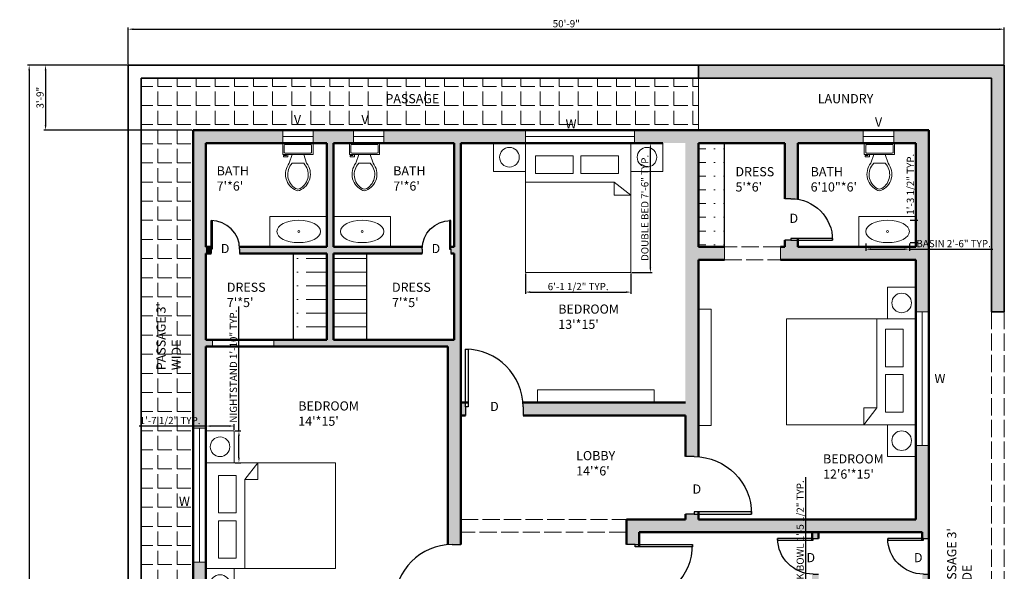
# Model space of a CAD drawing. Units: inches. Extents: x 554 to 1300, y 1707 to 2873.
# Tile 3 of 3: x 554 to 1238, y 2490 to 2873. Entities that reach past the tile are written whole.
import ezdxf

# ---------------------------------------------------------------- set-up
doc = ezdxf.new("R2010")
doc.units = ezdxf.units.IN
doc.linetypes.add('ACAD_ISO02W100', pattern=[15, 12, -3])
for name, color, linetype, lineweight in [('A-ANNO-DIMS', 145, 'Continuous', 18), ('A-AREA-IDEN', 145, 'Continuous', 25), ('A-CASE', 8, 'Continuous', 25), ('A-CASE-PATT', 245, 'Continuous', 13), ('A-FLOR-FIXT', 9, 'Continuous', 18), ('A-WALL-OVHD', 30, 'ACAD_ISO02W100', 18), ('A-WALL-PATT', 30, 'Continuous', 13), ('C-PROP', 30, 'Continuous', 35), ('C-PROP-OVHD', 30, 'ACAD_ISO02W100', 18), ('C-PVMT', 8, 'Continuous', 18), ('C-PVMT-PATT', 116, 'Continuous', 13), ('DOOR', 52, 'Continuous', 25), ('FUR', 210, 'Continuous', 18), ('TEXT', 145, 'Continuous', 18), ('WALL', 30, 'Continuous', 50), ('WIND', 70, 'Continuous', 18)]:
    doc.layers.add(name, color=color, linetype=linetype, lineweight=lineweight)
doc.styles.get("Standard").update_dxf_attribs({"font": 'arial.ttf'})
doc.dimstyles.new('ISO-25', dxfattribs={"dimtxt": 5, "dimasz": 3.5, "dimexe": 1.25, "dimexo": 0.625, "dimtad": 1, "dimdec": 0, "dimlunit": 4, "dimtxsty": 'Standard', "dimcen": 2.5, "dimadec": 0, "dimazin": 0, "dimtfac": 1, "dimtdec": 0, "dimtmove": 0, "dimatfit": 3, "dimfxl": 1, "dimarcsym": 0})

# ---------------------------------------------------------------- blocks, each defined once
blk = doc.blocks.new('*U2')
for p, q in [((0, 0), (0, -6)), ((40, 0), (40, -6))]:
    blk.add_line(p, q)
blk.add_lwpolyline([(0, 0), (0, 40), (1.75, 40), (1.75, 0)], close=True)
blk.add_arc((0, 0), 40, 0, 90)
blk = doc.blocks.new('*U4')
for p, q in [((9.5, -6), (9.5, -2)), ((-10, -8.5), (-8, -8.5)), ((-10, -9.5), (-10, -8.5)), ((-7, -9.5), (-10, -9.5)), ((-8, -8.5), (-8, -8)), ((-7, -8), (-7, -9.5)), ((-4, -8), (-6, -14)), ((4, -8), (6, -14)), ((4, -14), (-4, -14))]:
    blk.add_line(p, q)
blk.add_lwpolyline([(10.5, -8), (10.5, 0), (-10.5, 0), (-10.5, -8)], close=True)
for points in [[(-9.5, -2), (-9.5, -6)], [(8.5, -1), (-8.5, -1)], [(-8.5, -7), (8.5, -7)]]:
    blk.add_lwpolyline(points)
for centre, radius, start, end in [((-8.62, -1.88), 0.884, 81.8699, 188.1301), ((-8.62, -6.12), 0.884, 171.8699, 278.1301), ((8.62, -1.88), 0.884, 351.8699, 98.1301), ((8.62, -6.12), 0.884, 261.8699, 8.1301), ((3.52, -21.58), 12.17, 141.46911, 247.97143), ((4.2, -21.82), 11.33, 136.36773, 238.94682), ((-3.52, -21.58), 12.17, 292.02843, 38.53071), ((-4.2, -21.82), 11.33, 301.05301, 43.63209), ((0, -27.88), 4, 245.73182, 294.26817), ((0, -29), 4, 254.86053, 285.13947)]:
    blk.add_arc(centre, radius, start, end)
blk = doc.blocks.new('*D7')
at = {"layer": 'A-ANNO-DIMS', "color": 0, "lineweight": -2, "transparency": 16777216}
for p, q in [((629.68, 2842.1), (629.68, 2867.75)), ((633.18, 2866.5), (1234.68, 2866.5)), ((1238.18, 2842.1), (1238.18, 2867.75))]:
    blk.add_line(p, q, dxfattribs=at)
at = {"layer": 'A-ANNO-DIMS', "color": 0, "lineweight": 100, "transparency": 16777216}
for points in [[(633.18, 2867.08), (633.18, 2865.92), (629.68, 2866.5)], [(1234.68, 2867.08), (1234.68, 2865.92), (1238.18, 2866.5)]]:
    blk.add_solid(points, dxfattribs=at)
at = {"layer": 'Defpoints', "color": 0, "lineweight": 100, "transparency": 16777216}
for p in [(1238.18, 2866.5), (629.68, 2841.48), (1238.18, 2841.48)]:
    blk.add_point(p, dxfattribs=at)
at = {"layer": 'A-ANNO-DIMS', "color": 0, "transparency": 16777216, "insert": (933.93, 2869.68), "char_height": 5, "attachment_point": 5}
blk.add_mtext('50\'-9"', dxfattribs=at)
blk = doc.blocks.new('*D8')
at = {"layer": 'A-ANNO-DIMS', "color": 0, "lineweight": -2, "transparency": 16777216}
for p, q in [((629.06, 2841.48), (559.64, 2841.48)), ((560.89, 2837.98), (560.89, 1770.98)), ((629.06, 1767.48), (559.64, 1767.48))]:
    blk.add_line(p, q, dxfattribs=at)
at = {"layer": 'A-ANNO-DIMS', "color": 0, "lineweight": 100, "transparency": 16777216}
for points in [[(560.3, 2837.98), (561.47, 2837.98), (560.89, 2841.48)], [(560.3, 1770.98), (561.47, 1770.98), (560.89, 1767.48)]]:
    blk.add_solid(points, dxfattribs=at)
at = {"layer": 'Defpoints', "color": 0, "lineweight": 100, "transparency": 16777216}
for p in [(629.68, 2841.48), (560.89, 1767.48), (629.68, 1767.48)]:
    blk.add_point(p, dxfattribs=at)
at = {"layer": 'A-ANNO-DIMS', "color": 0, "transparency": 16777216, "insert": (557.71, 2304.48), "char_height": 5, "attachment_point": 5, "rotation": 90}
blk.add_mtext('89\'-6"', dxfattribs=at)
blk = doc.blocks.new('BED-DOUBLE')
for p, q in [((0, 62.82), (61.67, 62.82)), ((61.67, 62.82), (61.67, 53.82)), ((73.37, 53.82), (61.67, 62.82)), ((61.67, 53.82), (73.37, 53.82))]:
    blk.add_line(p, q)
blk.add_lwpolyline([(73.37, 89.87), (73.37, 0), (0, 0), (0, 89.87)])
for points in [[(7.06, 81.16), (33.12, 81.16), (33.12, 68.85), (7.06, 68.85)], [(38.57, 81.16), (64.63, 81.16), (64.63, 68.85), (38.57, 68.85)]]:
    blk.add_lwpolyline(points, close=True)
blk = doc.blocks.new('NIGHTSTAND')
blk.add_lwpolyline([(22.14, 19.58), (0, 19.58), (0, 0), (22.14, 0)], close=True)
blk.add_circle((11.07, 9.79), 6.79)
blk = doc.blocks.new('BASIN-OVAL')
blk.add_circle((15.12, 7.78), 0.687)
blk.add_ellipse((15.12, 7.78), major_axis=(15.12, 0), ratio=0.514491)
blk = doc.blocks.new('*D18')
at = {"layer": 'A-ANNO-DIMS', "color": 0, "lineweight": -2, "transparency": 16777216}
for p, q in [((706.58, 2587.89), (706.58, 2674.1)), ((703.88, 2587.89), (707.83, 2587.89)), ((706.58, 2569.25), (706.58, 2584.39)), ((703.88, 2565.75), (707.83, 2565.75))]:
    blk.add_line(p, q, dxfattribs=at)
at = {"layer": 'A-ANNO-DIMS', "color": 0, "lineweight": 100, "transparency": 16777216}
for points in [[(706, 2584.39), (707.16, 2584.39), (706.58, 2587.89)], [(706, 2569.25), (707.16, 2569.25), (706.58, 2565.75)]]:
    blk.add_solid(points, dxfattribs=at)
at = {"layer": 'Defpoints', "color": 0, "lineweight": 100, "transparency": 16777216}
for p in [(703.26, 2587.89), (706.58, 2587.89), (703.26, 2565.75)]:
    blk.add_point(p, dxfattribs=at)
at = {"layer": 'A-ANNO-DIMS', "color": 0, "transparency": 16777216, "insert": (703.37, 2632.74), "char_height": 5, "attachment_point": 5, "rotation": 90}
blk.add_mtext('NIGHTSTAND 1\'-10" TYP.', dxfattribs=at)
blk = doc.blocks.new('*D19')
at = {"layer": 'A-ANNO-DIMS', "color": 0, "lineweight": -2, "transparency": 16777216}
for p, q in [((683.68, 2588.51), (683.68, 2592.46)), ((703.26, 2588.51), (703.26, 2592.46)), ((683.68, 2591.21), (637.27, 2591.21)), ((699.76, 2591.21), (687.18, 2591.21))]:
    blk.add_line(p, q, dxfattribs=at)
at = {"layer": 'A-ANNO-DIMS', "color": 0, "lineweight": 100, "transparency": 16777216}
for points in [[(687.18, 2591.79), (687.18, 2590.62), (683.68, 2591.21)], [(699.76, 2591.79), (699.76, 2590.62), (703.26, 2591.21)]]:
    blk.add_solid(points, dxfattribs=at)
at = {"layer": 'Defpoints', "color": 0, "lineweight": 100, "transparency": 16777216}
for p in [(683.68, 2591.21), (683.68, 2587.89), (703.26, 2587.89)]:
    blk.add_point(p, dxfattribs=at)
at = {"layer": 'A-ANNO-DIMS', "color": 0, "transparency": 16777216, "insert": (658.73, 2594.42), "char_height": 5, "attachment_point": 5}
blk.add_mtext('1\'-7 1/2" TYP.', dxfattribs=at)
blk = doc.blocks.new('*D22')
at = {"layer": 'A-ANNO-DIMS', "color": 0, "lineweight": -2, "transparency": 16777216}
for p, q in [((1142.01, 2717.81), (1142.01, 2712.65)), ((1172.26, 2717.81), (1172.26, 2712.65)), ((1145.51, 2713.9), (1168.76, 2713.9)), ((1172.26, 2713.9), (1230.16, 2713.9))]:
    blk.add_line(p, q, dxfattribs=at)
at = {"layer": 'A-ANNO-DIMS', "color": 0, "lineweight": 100, "transparency": 16777216}
for points in [[(1145.51, 2714.48), (1145.51, 2713.32), (1142.01, 2713.9)], [(1168.76, 2714.48), (1168.76, 2713.32), (1172.26, 2713.9)]]:
    blk.add_solid(points, dxfattribs=at)
at = {"layer": 'Defpoints', "color": 0, "lineweight": 100, "transparency": 16777216}
for p in [(1142.01, 2718.44), (1172.26, 2718.44), (1172.26, 2713.9)]:
    blk.add_point(p, dxfattribs=at)
at = {"layer": 'A-ANNO-DIMS', "color": 0, "transparency": 16777216, "insert": (1202.96, 2717.11), "char_height": 5, "attachment_point": 5}
blk.add_mtext('BASIN 2\'-6" TYP.', dxfattribs=at)
blk = doc.blocks.new('*D23')
at = {"layer": 'A-ANNO-DIMS', "color": 0, "lineweight": -2, "transparency": 16777216}
for p, q in [((1176.79, 2734), (1176.79, 2780.41)), ((1172.88, 2734), (1178.04, 2734)), ((1176.79, 2721.94), (1176.79, 2730.5)), ((1172.88, 2718.44), (1178.04, 2718.44))]:
    blk.add_line(p, q, dxfattribs=at)
at = {"layer": 'A-ANNO-DIMS', "color": 0, "lineweight": 100, "transparency": 16777216}
for points in [[(1176.21, 2730.5), (1177.38, 2730.5), (1176.79, 2734)], [(1176.21, 2721.94), (1177.38, 2721.94), (1176.79, 2718.44)]]:
    blk.add_solid(points, dxfattribs=at)
at = {"layer": 'Defpoints', "color": 0, "lineweight": 100, "transparency": 16777216}
for p in [(1172.26, 2734), (1176.79, 2734), (1172.26, 2718.44)]:
    blk.add_point(p, dxfattribs=at)
at = {"layer": 'A-ANNO-DIMS', "color": 0, "transparency": 16777216, "insert": (1173.58, 2758.95), "char_height": 5, "attachment_point": 5, "rotation": 90}
blk.add_mtext('1\'-3 1/2" TYP.', dxfattribs=at)
blk = doc.blocks.new('*D24')
at = {"layer": 'A-ANNO-DIMS', "color": 0, "lineweight": -2, "transparency": 16777216}
for p, q in [((979.52, 2787.48), (993.62, 2787.48)), ((992.37, 2701.11), (992.37, 2783.98)), ((979.52, 2697.61), (993.62, 2697.61))]:
    blk.add_line(p, q, dxfattribs=at)
at = {"layer": 'A-ANNO-DIMS', "color": 0, "lineweight": 100, "transparency": 16777216}
for points in [[(991.79, 2783.98), (992.96, 2783.98), (992.37, 2787.48)], [(991.79, 2701.11), (992.96, 2701.11), (992.37, 2697.61)]]:
    blk.add_solid(points, dxfattribs=at)
at = {"layer": 'Defpoints', "color": 0, "lineweight": 100, "transparency": 16777216}
for p in [(978.89, 2787.48), (992.37, 2787.48), (978.89, 2697.61)]:
    blk.add_point(p, dxfattribs=at)
at = {"layer": 'A-ANNO-DIMS', "color": 0, "transparency": 16777216, "insert": (989.16, 2742.54), "char_height": 5, "attachment_point": 5, "rotation": 90}
blk.add_mtext('DOUBLE BED 7\'-6" TYP.', dxfattribs=at)
blk = doc.blocks.new('*D25')
at = {"layer": 'A-ANNO-DIMS', "color": 0, "lineweight": -2, "transparency": 16777216}
for p, q in [((905.53, 2696.98), (905.53, 2682.87)), ((978.89, 2696.98), (978.89, 2682.87)), ((909.03, 2684.12), (975.39, 2684.12))]:
    blk.add_line(p, q, dxfattribs=at)
at = {"layer": 'A-ANNO-DIMS', "color": 0, "lineweight": 100, "transparency": 16777216}
for points in [[(909.03, 2684.71), (909.03, 2683.54), (905.53, 2684.12)], [(975.39, 2684.71), (975.39, 2683.54), (978.89, 2684.12)]]:
    blk.add_solid(points, dxfattribs=at)
at = {"layer": 'Defpoints', "color": 0, "lineweight": 100, "transparency": 16777216}
for p in [(905.53, 2697.61), (978.89, 2697.61), (978.89, 2684.12)]:
    blk.add_point(p, dxfattribs=at)
at = {"layer": 'A-ANNO-DIMS', "color": 0, "transparency": 16777216, "insert": (942.21, 2687.33), "char_height": 5, "attachment_point": 5}
blk.add_mtext('6\'-1 1/2" TYP.', dxfattribs=at)
blk = doc.blocks.new('*D28')
at = {"layer": 'A-ANNO-DIMS', "color": 0, "lineweight": -2, "transparency": 16777216}
for p, q in [((1100.29, 2468.04), (1100.29, 2555.65)), ((1098.27, 2468.04), (1101.54, 2468.04)), ((1100.29, 2453.96), (1100.29, 2464.54)), ((1098.27, 2450.46), (1101.54, 2450.46))]:
    blk.add_line(p, q, dxfattribs=at)
at = {"layer": 'A-ANNO-DIMS', "color": 0, "lineweight": 100, "transparency": 16777216}
for points in [[(1099.7, 2464.54), (1100.87, 2464.54), (1100.29, 2468.04)], [(1099.7, 2453.96), (1100.87, 2453.96), (1100.29, 2450.46)]]:
    blk.add_solid(points, dxfattribs=at)
at = {"layer": 'Defpoints', "color": 0, "lineweight": 100, "transparency": 16777216}
for p in [(1097.65, 2468.04), (1100.29, 2468.04), (1097.65, 2450.46)]:
    blk.add_point(p, dxfattribs=at)
at = {"layer": 'A-ANNO-DIMS', "color": 0, "transparency": 16777216, "insert": (1097.07, 2513.59), "char_height": 5, "attachment_point": 5, "rotation": 90}
blk.add_mtext('SINK BOWL 1\'-5 1/2" TYP.', dxfattribs=at)
blk = doc.blocks.new('*D35')
at = {"layer": 'A-ANNO-DIMS', "color": 0, "lineweight": -2, "transparency": 16777216}
for p, q in [((629.06, 2841.48), (571.03, 2841.48)), ((572.28, 2837.98), (572.28, 2799.98)), ((674.06, 2796.48), (571.03, 2796.48))]:
    blk.add_line(p, q, dxfattribs=at)
at = {"layer": 'A-ANNO-DIMS', "color": 0, "lineweight": 100, "transparency": 16777216}
for points in [[(571.7, 2837.98), (572.86, 2837.98), (572.28, 2841.48)], [(571.7, 2799.98), (572.86, 2799.98), (572.28, 2796.48)]]:
    blk.add_solid(points, dxfattribs=at)
at = {"layer": 'Defpoints', "color": 0, "lineweight": 100, "transparency": 16777216}
for p in [(629.68, 2841.48), (572.28, 2796.48), (674.68, 2796.48)]:
    blk.add_point(p, dxfattribs=at)
at = {"layer": 'A-ANNO-DIMS', "color": 0, "transparency": 16777216, "insert": (569.1, 2818.98), "char_height": 5, "attachment_point": 5, "rotation": 90}
blk.add_mtext('3\'-9"', dxfattribs=at)

msp = doc.modelspace()

# ---------------------------------------------------------------- hatches: boundary and pattern name
at = {"layer": 'A-CASE-PATT'}
h = msp.add_hatch(dxfattribs=at)
h.set_pattern_fill('ACAD_ISO04W100', color=256, scale=1.9)
h.paths.add_polyline_path([(767.68, 2710.98), (744.53, 2710.98), (744.53, 2650.98), (767.68, 2650.98)])
h.paths.add_polyline_path([(795.22, 2710.98), (772.18, 2710.98), (772.18, 2650.98), (795.22, 2650.98)])
h.paths.add_polyline_path([(1043.78, 2787.48), (1025.68, 2787.48), (1025.68, 2715.48), (1043.78, 2715.48)])
at = {"layer": 'A-WALL-PATT'}
h = msp.add_hatch(color=256, dxfattribs=at)
h.dxf.hatch_style = 1
h.paths.add_polyline_path([(1238.18, 2841.48), (1025.68, 2841.48), (1025.68, 2832.48), (1229.18, 2832.48), (1229.18, 2670.52), (1238.18, 2670.52)])
h = msp.add_hatch(color=256, dxfattribs=at)
h.dxf.hatch_style = 1
h.paths.add_polyline_path([(1136.18, 2067.48), (1026.18, 2067.48), (1026.18, 2065.48), (1134.18, 2065.48), (1134.18, 2039.48), (1026.18, 2039.48), (1026.18, 2037.48), (1136.18, 2037.48)])
h.paths.add_polyline_path([(1193.18, 2103.48), (1184.18, 2103.48), (1184.18, 2077.52), (1193.18, 2077.52)])
h.paths.add_polyline_path([(1193.18, 2032.94), (1184.18, 2032.94), (1184.18, 2001.48), (1148.18, 2001.48), (1136.18, 2001.48), (1128.74, 2001.48), (1128.74, 1992.48), (1193.18, 1992.48), (1193.18, 2001.48)])
h.paths.add_polyline_path([(1076.18, 2001.48), (1045.59, 2001.48), (1045.59, 1992.48), (1076.18, 1992.48)])
h.paths.add_polyline_path([(993.02, 2001.48), (923.53, 2001.48), (923.53, 1996.9), (923.53, 1992.48), (993.02, 1992.48)])
h.paths.add_polyline_path([(1184.18, 2112.48), (962.18, 2112.48), (962.18, 2151.15), (953.18, 2151.15), (953.18, 2103.48), (1184.18, 2103.48)])
h.paths.add_polyline_path([(1193.18, 2144.33), (1184.18, 2144.33), (1184.18, 2112.48), (1184.18, 2103.48), (1193.18, 2103.48)])
h.paths.add_polyline_path([(772.18, 2796.48), (758.22, 2796.48), (758.22, 2787.48), (767.68, 2787.48), (772.18, 2787.48)])
h.paths.add_polyline_path([(737.06, 2796.48), (674.68, 2796.48), (674.68, 2710.98), (683.68, 2710.98), (683.68, 2715.48), (683.68, 2787.48), (737.06, 2787.48)])
h.paths.add_polyline_path([(786.15, 2796.48), (772.18, 2796.48), (772.18, 2787.48), (786.15, 2787.48)])
h.paths.add_polyline_path([(860.68, 2796.48), (807.31, 2796.48), (807.31, 2787.48), (856.18, 2787.48), (860.68, 2787.48)])
h.paths.add_polyline_path([(905.53, 2796.48), (860.68, 2796.48), (860.68, 2787.48), (905.53, 2787.48)])
h.paths.add_polyline_path([(860.68, 2787.48), (856.18, 2787.48), (856.18, 2715.48), (853.67, 2715.48), (853.67, 2713.96), (853.67, 2710.98), (856.18, 2710.98), (860.68, 2710.98)])
h.paths.add_polyline_path([(772.18, 2787.48), (767.68, 2787.48), (767.68, 2715.48), (728.12, 2715.48), (706.98, 2715.48, -0.019152), (707.04, 2713.96), (707.04, 2710.98), (772.18, 2710.98)])
h.paths.add_polyline_path([(833.86, 2715.48), (772.18, 2715.48), (772.18, 2710.98), (833.8, 2710.98), (833.8, 2713.96, -0.019152)])
h.paths.add_polyline_path([(1025.68, 2796.48), (981.39, 2796.48), (981.39, 2787.48), (1001.03, 2787.48), (1016.68, 2787.48), (1025.68, 2787.48)])
h.paths.add_polyline_path([(1094.68, 2796.48), (1025.68, 2796.48), (1025.68, 2787.48), (1085.68, 2787.48), (1094.68, 2787.48)])
h.paths.add_polyline_path([(1140.18, 2796.48), (1094.68, 2796.48), (1094.68, 2787.48), (1140.18, 2787.48)], flags=17)
h.paths.add_polyline_path([(1185.68, 2796.48), (1161.35, 2796.48), (1161.35, 2787.48), (1176.68, 2787.48), (1176.68, 2736.68), (1176.72, 2736.68), (1176.72, 2715.48), (1137.16, 2715.48), (1094.68, 2715.48), (1094.68, 2706.48), (1185.68, 2706.48)])
h.paths.add_polyline_path([(1094.68, 2787.48), (1085.68, 2787.48), (1085.68, 2748.92), (1090.01, 2748.92, -0.040642), (1094.68, 2748.54)])
h.paths.add_polyline_path([(1025.68, 2787.48), (1016.68, 2787.48), (1016.68, 2607.48), (1016.68, 2598.48), (1025.68, 2598.48), (1025.68, 2672.36), (1025.68, 2706.48)])
h.paths.add_polyline_path([(1094.68, 2715.48), (1094.68, 2720.05), (1090.01, 2720.05), (1085.68, 2720.05), (1085.68, 2715.48), (1082.66, 2715.48), (1082.66, 2706.48), (1094.68, 2706.48)])
h.paths.add_polyline_path([(1043.78, 2715.48), (1025.68, 2715.48), (1025.68, 2706.48), (1043.78, 2706.48)])
h.paths.add_polyline_path([(1185.68, 2577.7), (1176.68, 2577.7), (1176.68, 2570), (1176.68, 2526.48), (1176.68, 2517.48), (1185.68, 2517.48)])
h.paths.add_polyline_path([(1185.68, 2706.48), (1176.68, 2706.48), (1176.68, 2670.52), (1185.68, 2670.52)])
h.paths.add_polyline_path([(1025.68, 2598.48), (1016.68, 2598.48), (1016.68, 2569.99), (1022.68, 2569.99, -0.01877), (1025.68, 2569.88)])
h.paths.add_polyline_path([(1016.68, 2607.48), (903.83, 2607.48, -0.01877), (903.94, 2604.48), (903.94, 2598.48), (1016.68, 2598.48)])
h.paths.add_polyline_path([(860.68, 2646.48), (851.68, 2646.48), (851.68, 2508.85, -0.01877), (854.68, 2508.96), (860.68, 2508.96)])
h.paths.add_polyline_path([(863.94, 2604.48), (863.94, 2607.48), (860.68, 2607.48), (860.68, 2598.48), (863.94, 2598.48)])
h.paths.add_polyline_path([(1101.44, 2750.41), (1134.65, 2750.41), (1134.65, 2774.1), (1101.44, 2774.1)], flags=25)
h.paths.add_polyline_path([(1049.21, 2750.31), (1082.94, 2750.31), (1082.94, 2773.99), (1049.21, 2773.99)], flags=9)
h = msp.add_hatch(color=256, dxfattribs=at)
h.dxf.hatch_style = 1
h.paths.add_polyline_path([(687.18, 2713.96), (687.18, 2715.48), (683.68, 2715.48), (683.68, 2710.98), (687.18, 2710.98)])
h = msp.add_hatch(color=256, dxfattribs=at)
h.dxf.hatch_style = 1
h.paths.add_polyline_path([(683.68, 2710.98), (674.68, 2710.98), (674.68, 2646.48), (674.68, 2589.67), (683.68, 2589.67), (683.68, 2646.48), (683.68, 2650.98)])
h.paths.add_polyline_path([(688.17, 2650.98), (683.68, 2650.98), (683.68, 2646.48), (688.17, 2646.48)])
h.paths.add_polyline_path([(772.18, 2710.98), (767.68, 2710.98), (767.68, 2650.98), (730.85, 2650.98), (730.85, 2646.48), (772.18, 2646.48)])
h.paths.add_polyline_path([(860.68, 2710.98), (856.18, 2710.98), (856.18, 2650.98), (772.18, 2650.98), (772.18, 2646.48), (860.68, 2646.48)])
h.paths.add_polyline_path([(683.68, 2496.84), (674.68, 2496.84), (674.68, 2445.48), (683.68, 2445.48), (683.68, 2454.48)])
h.paths.add_polyline_path([(851.68, 2454.48), (683.68, 2454.48), (683.68, 2445.48), (851.68, 2445.48)])
h.paths.add_polyline_path([(707.68, 2445.48), (698.68, 2445.48), (698.68, 2419.1), (707.68, 2419.1)])
h.paths.add_polyline_path([(698.68, 2289.48), (687.57, 2289.48), (687.57, 2280.48), (696.57, 2280.48), (698.68, 2280.48)])
h.paths.add_polyline_path([(687.57, 2217.48), (671.17, 2217.48), (671.17, 2208.48), (687.57, 2208.48)])
h.paths.add_polyline_path([(650.01, 2217.48), (638.68, 2217.48), (638.68, 2208.48), (650.01, 2208.48)])
h.paths.add_polyline_path([(860.68, 2235.34), (854.68, 2235.34, -0.01877), (851.68, 2235.45), (851.68, 2112.48), (696.57, 2112.48), (696.57, 2103.48), (860.68, 2103.48)])
h.paths.add_polyline_path([(666.88, 1959.48), (647.68, 1959.48), (638.68, 1959.48), (638.68, 1950.48), (647.68, 1950.48), (666.88, 1950.48)])
h.paths.add_polyline_path([(756.66, 1959.48), (719.44, 1959.48), (719.44, 1950.48), (756.66, 1950.48)])
h.paths.add_polyline_path([(860.68, 1992.48), (864.62, 1992.48), (864.62, 1996.9), (864.62, 2001.48), (860.68, 2001.48), (860.68, 2058.13), (854.68, 2058.13, -0.01877), (851.68, 2058.24), (851.68, 1992.48), (851.68, 1959.48), (809.22, 1959.48), (809.22, 1950.48), (860.68, 1950.48)])
h.paths.add_polyline_path([(860.68, 2103.48), (851.68, 2103.48), (851.68, 2098.13), (854.68, 2098.13), (860.68, 2098.13)])
h.paths.add_polyline_path([(984.68, 2397.2), (984.68, 2469.19, -0.01877), (981.68, 2469.08), (975.68, 2469.08), (975.68, 2361.48), (975.68, 2355.65), (984.68, 2355.65), (984.68, 2361.48), (984.68, 2370.48)])
h.paths.add_polyline_path([(1109.18, 2409.48), (1104.68, 2409.48), (1104.68, 2370.48), (984.68, 2370.48), (984.68, 2361.48), (1109.18, 2361.48)])
h.paths.add_polyline_path([(1125.26, 2418.48), (1109.18, 2418.48), (1109.18, 2488.51), (1105.47, 2488.51, -0.008003), (1104.68, 2488.52), (1104.68, 2409.48), (1109.18, 2409.48), (1125.26, 2409.48)])
h.paths.add_polyline_path([(1185.68, 2418.48), (1167, 2418.48), (1167, 2409.48), (1185.68, 2409.48)])
h.paths.add_polyline_path([(1185.68, 2488.51), (1181.97, 2488.51, -0.008003), (1181.18, 2488.52), (1181.18, 2418.48), (1185.68, 2418.48)])
h.paths.add_polyline_path([(1025.68, 2529.99), (1022.68, 2529.99), (1016.68, 2529.99), (1016.68, 2526.48), (975.68, 2526.48), (975.68, 2517.48), (1025.68, 2517.48)])
h.paths.add_polyline_path([(984.68, 2517.48), (975.68, 2517.48), (975.68, 2509.08), (981.68, 2509.08), (984.68, 2509.08)])
h.paths.add_polyline_path([(1176.68, 2526.48), (1025.68, 2526.48), (1025.68, 2517.48), (1104.68, 2517.48), (1176.68, 2517.48)])
h.paths.add_polyline_path([(745.17, 1864.25), (773.96, 1864.25), (773.96, 1877.33), (745.17, 1877.33)], flags=9)
h = msp.add_hatch(color=256, dxfattribs=at)
h.dxf.hatch_style = 1
h.paths.add_polyline_path([(638.68, 2072.33), (638.68, 2103.48), (638.68, 2217.48), (629.68, 2217.48), (629.68, 2097.48), (629.68, 1992.48), (629.68, 1950.48), (638.68, 1950.48), (638.68, 1992.48)])
h.paths.add_polyline_path([(696.57, 2217.48), (687.57, 2217.48), (687.57, 2142.07, -0.048021), (692.61, 2142.55), (696.57, 2142.55)])
h.paths.add_polyline_path([(696.57, 2116.14), (692.61, 2116.14), (687.57, 2116.14), (687.57, 2112.48), (638.68, 2112.48), (638.68, 2103.48), (687.57, 2103.48), (696.57, 2103.48), (696.57, 2112.48)])
h.paths.add_polyline_path([(1010.14, 2078.06), (1025.63, 2078.06), (1025.63, 2091.14), (1010.14, 2091.14)], flags=9)
h.paths.add_polyline_path([(1129.91, 2440.07), (1172.04, 2440.07), (1172.04, 2474.45), (1129.91, 2474.45)], flags=9)
h.paths.add_polyline_path([(1022.04, 2432.2), (1064.45, 2432.2), (1064.45, 2455.89), (1022.04, 2455.89)], flags=9)
h.paths.add_polyline_path([(891.25, 2147.87), (936.31, 2147.87), (936.31, 2182.23), (891.25, 2182.23)], flags=9)
h.paths.add_polyline_path([(951.1, 2040.21), (1005.03, 2040.21), (1005.03, 2063.9), (951.1, 2063.9)], flags=9)
h.paths.add_polyline_path([(988, 1912.76), (1023.48, 1912.76), (1023.48, 1936.45), (988, 1936.45)], flags=9)
h.paths.add_polyline_path([(735.06, 2044.01), (781.37, 2044.01), (781.37, 2078.39), (735.06, 2078.39)], flags=9)
h.paths.add_polyline_path([(651.07, 2140.85), (677.89, 2140.85), (677.89, 2164.54), (651.07, 2164.54)], flags=9)
h.paths.add_polyline_path([(769.16, 2219.79), (818.47, 2219.79), (818.47, 2243.48), (769.16, 2243.48)], flags=9)
h.paths.add_polyline_path([(745.28, 2587.79), (794.59, 2587.79), (794.59, 2611.48), (745.28, 2611.48)], flags=9)
h = msp.add_hatch(color=256, dxfattribs=at)
h.dxf.hatch_style = 1
h.paths.add_polyline_path([(1109.18, 2517.48), (1104.68, 2517.48), (1104.68, 2513.23), (1105.47, 2513.23), (1109.18, 2513.23)])
h.paths.add_polyline_path([(1185.68, 2517.48), (1181.18, 2517.48), (1181.18, 2513.23), (1181.97, 2513.23), (1185.68, 2513.23)])
at = {"layer": 'C-PVMT-PATT'}
h = msp.add_hatch(dxfattribs=at)
h.set_pattern_fill('ANGLE', color=256, scale=1.9)
h.set_pattern_definition([(0, (0, 0), (0, 13.2715), [9.652, -3.6195]), (90, (0, 0), (-13.2715, 8e-16), [9.652, -3.6195])])
h.paths.add_polyline_path([(674.68, 2646.48), (674.68, 2710.98), (674.68, 2796.48), (772.18, 2796.48), (860.68, 2796.48), (1025.68, 2796.48), (1025.68, 2832.48), (638.68, 2832.48), (638.68, 2217.48), (674.68, 2217.48), (674.68, 2445.48)])

# ---------------------------------------------------------------- linework, layer by layer
at = {"layer": 'A-CASE'}
for p, q in [((1043.78, 2715.48), (1043.78, 2787.48)), ((744.53, 2650.98), (744.53, 2710.98)), ((795.22, 2710.98), (795.22, 2650.98))]:
    msp.add_line(p, q, dxfattribs=at)
at = {"layer": 'A-FLOR-FIXT'}
for points in [[(767.68, 2715.48), (728.12, 2715.48), (728.12, 2736.68), (767.68, 2736.68)], [(811.74, 2715.48), (772.18, 2715.48), (772.18, 2736.68), (811.74, 2736.68)], [(1176.72, 2715.48), (1137.16, 2715.48), (1137.16, 2736.68), (1176.72, 2736.68)]]:
    msp.add_lwpolyline(points, close=True, dxfattribs=at)
at = {"layer": 'A-WALL-OVHD'}
for points in [[(1043.78, 2706.48), (1043.78, 2715.48)], [(1082.66, 2715.48), (1082.66, 2706.48)]]:
    msp.add_lwpolyline(points, dxfattribs=at)
for points in [[(1043.78, 2706.48), (1082.66, 2706.48), (1082.66, 2715.48), (1043.78, 2715.48)], [(688.17, 2650.98), (730.85, 2650.98), (730.85, 2646.48), (688.17, 2646.48)], [(975.68, 2517.48), (860.68, 2517.48), (860.68, 2526.48), (975.68, 2526.48)]]:
    msp.add_lwpolyline(points, close=True, dxfattribs=at)
at = {"layer": 'C-PROP'}
for p, q in [((629.68, 2841.48), (629.68, 2097.48)), ((629.68, 2841.48), (1238.18, 2841.48)), ((1025.68, 2832.48), (1025.68, 2841.48)), ((1238.18, 2670.52), (1238.18, 2841.48)), ((638.68, 2832.48), (1229.18, 2832.48)), ((638.68, 2832.48), (638.68, 2097.48)), ((1229.18, 2670.52), (1229.18, 2832.48)), ((1229.18, 2670.52), (1238.18, 2670.52))]:
    msp.add_line(p, q, dxfattribs=at)
at = {"layer": 'C-PROP-OVHD'}
msp.add_lwpolyline([(1229.18, 2418.48), (1238.18, 2418.48), (1238.18, 2670.52), (1229.18, 2670.52)], close=True, dxfattribs=at)
at = {"layer": 'C-PVMT'}
msp.add_line((1025.68, 2796.48), (1025.68, 2832.48), dxfattribs=at)
at = {"layer": 'FUR'}
for p, q in [((719.73, 2565.75), (710.74, 2554.05)), ((719.73, 2554.05), (719.73, 2565.75)), ((710.74, 2492.38), (710.74, 2554.05)), ((710.74, 2554.05), (719.73, 2554.05))]:
    msp.add_line(p, q, dxfattribs=at)
for points in [[(1001.03, 2787.48), (978.89, 2787.48), (978.89, 2767.9), (1001.03, 2767.9)], [(1025.68, 2672.36), (1025.68, 2591.51), (1034.61, 2591.51), (1034.61, 2672.36)], [(914.03, 2607.48), (994.88, 2607.48), (994.88, 2616.41), (914.03, 2616.41)], [(1176.68, 2570), (1176.68, 2592.14), (1157.1, 2592.14), (1157.1, 2570)], [(692.39, 2530.95), (692.39, 2557.01), (704.7, 2557.01), (704.7, 2530.95)], [(692.39, 2499.44), (692.39, 2525.5), (704.7, 2525.5), (704.7, 2499.44)]]:
    msp.add_lwpolyline(points, close=True, dxfattribs=at)
msp.add_lwpolyline([(683.68, 2565.75), (773.56, 2565.75), (773.56, 2492.38), (683.68, 2492.38), (683.68, 2496.84)], dxfattribs=at)
for centre in [(989.96, 2777.69), (1166.89, 2581.07)]:
    msp.add_circle(centre, 6.79, dxfattribs=at)
at = {"layer": 'WALL'}
for p, q in [((674.68, 2796.48), (772.18, 2796.48)), ((674.68, 2710.98), (674.68, 2796.48)), ((772.18, 2796.48), (860.68, 2796.48)), ((860.68, 2796.48), (1025.68, 2796.48)), ((1025.68, 2796.48), (1094.68, 2796.48)), ((1094.68, 2796.48), (1185.68, 2796.48)), ((1185.68, 2796.48), (1185.68, 2706.48)), ((683.68, 2787.48), (767.68, 2787.48)), ((683.68, 2715.48), (683.68, 2787.48)), ((767.68, 2787.48), (767.68, 2715.48)), ((772.18, 2787.48), (772.18, 2715.48)), ((772.18, 2787.48), (856.18, 2787.48)), ((856.18, 2787.48), (856.18, 2715.48)), ((860.68, 2787.48), (860.68, 2710.98)), ((860.68, 2787.48), (1001.03, 2787.48)), ((1025.68, 2787.48), (1025.68, 2715.48)), ((1025.68, 2787.48), (1085.68, 2787.48)), ((1085.68, 2787.48), (1085.68, 2748.92)), ((1094.68, 2787.48), (1094.68, 2748.54)), ((1094.68, 2787.48), (1176.68, 2787.48)), ((1176.68, 2787.48), (1176.68, 2715.48)), ((688.05, 2715.48), (683.68, 2715.48)), ((767.68, 2715.48), (706.98, 2715.48)), ((833.86, 2715.48), (772.18, 2715.48)), ((856.18, 2715.48), (852.8, 2715.48)), ((1043.78, 2715.48), (1025.68, 2715.48)), ((1085.68, 2715.48), (1082.66, 2715.48)), ((1085.68, 2720.05), (1085.68, 2715.48)), ((1094.68, 2721.31), (1094.68, 2715.48)), ((1176.68, 2715.48), (1094.68, 2715.48)), ((674.68, 2710.98), (674.68, 2646.48)), ((683.68, 2710.98), (683.68, 2650.98)), ((687.18, 2710.98), (683.68, 2710.98)), ((767.68, 2710.98), (707.04, 2710.98)), ((767.68, 2650.98), (767.68, 2710.98)), ((772.18, 2650.98), (772.18, 2710.98)), ((772.18, 2710.98), (833.8, 2710.98)), ((833.8, 2710.98), (772.18, 2710.98)), ((856.18, 2710.98), (853.67, 2710.98)), ((853.67, 2710.98), (856.18, 2710.98)), ((856.18, 2710.98), (856.18, 2650.98)), ((860.68, 2710.98), (860.68, 2646.48)), ((1025.68, 2706.48), (1025.68, 2569.88)), ((1043.78, 2706.48), (1025.68, 2706.48)), ((1025.68, 2706.48), (1025.68, 2598.48)), ((1094.68, 2706.48), (1082.66, 2706.48)), ((1176.68, 2706.48), (1094.68, 2706.48)), ((1176.68, 2526.48), (1176.68, 2706.48)), ((1185.68, 2517.48), (1185.68, 2706.48)), ((683.68, 2650.98), (767.68, 2650.98)), ((856.18, 2650.98), (772.18, 2650.98)), ((674.68, 2646.48), (674.68, 2445.48)), ((683.68, 2646.48), (772.18, 2646.48)), ((683.68, 2646.48), (683.68, 2454.48)), ((851.68, 2646.48), (772.18, 2646.48)), ((851.68, 2508.85), (851.68, 2646.48)), ((860.68, 2508.96), (860.68, 2646.48)), ((865.69, 2607.48), (860.68, 2607.48)), ((1016.68, 2607.48), (903.83, 2607.48)), ((860.68, 2598.48), (860.68, 2526.48)), ((863.94, 2598.48), (860.68, 2598.48)), ((1016.68, 2598.48), (903.94, 2598.48)), ((1016.68, 2598.48), (1016.68, 2569.99)), ((1025.68, 2598.48), (1025.68, 2569.88)), ((1025.68, 2531.74), (1025.68, 2526.48)), ((1025.68, 2531.74), (1025.68, 2526.48)), ((1016.68, 2526.48), (975.68, 2526.48)), ((975.68, 2517.48), (975.68, 2526.48)), ((1016.68, 2529.99), (1016.68, 2526.48)), ((1025.68, 2526.48), (1176.68, 2526.48)), ((975.68, 2517.48), (975.68, 2509.08)), ((1025.68, 2517.48), (984.68, 2517.48)), ((1104.68, 2517.48), (984.68, 2517.48)), ((984.68, 2517.48), (984.68, 2507.33)), ((1025.68, 2517.48), (1181.18, 2517.48)), ((1104.68, 2512.15), (1104.68, 2517.48)), ((1109.18, 2513.23), (1109.18, 2517.48)), ((1181.18, 2517.48), (1181.18, 2512.15)), ((1185.68, 2517.48), (1185.68, 2418.48))]:
    msp.add_line(p, q, dxfattribs=at)
at = {"layer": 'WIND'}
for p, q in [((737.06, 2791.98), (758.22, 2791.98)), ((786.15, 2791.98), (807.31, 2791.98)), ((905.53, 2791.98), (981.39, 2791.98)), ((1140.18, 2791.98), (1161.35, 2791.98)), ((1181.18, 2577.7), (1181.18, 2670.52)), ((679.18, 2496.84), (679.18, 2589.67))]:
    msp.add_line(p, q, dxfattribs=at)
for points in [[(737.06, 2787.48), (758.22, 2787.48), (758.22, 2796.48), (737.06, 2796.48)], [(786.15, 2787.48), (807.31, 2787.48), (807.31, 2796.48), (786.15, 2796.48)], [(905.53, 2796.48), (981.39, 2796.48), (981.39, 2787.48), (905.53, 2787.48)], [(1140.18, 2787.48), (1161.35, 2787.48), (1161.35, 2796.48), (1140.18, 2796.48)], [(1176.68, 2670.52), (1185.68, 2670.52), (1185.68, 2577.7), (1176.68, 2577.7)], [(674.68, 2589.67), (683.68, 2589.67), (683.68, 2496.84), (674.68, 2496.84)]]:
    msp.add_lwpolyline(points, close=True, dxfattribs=at)

# ---------------------------------------------------------------- block references
at = {"layer": 'A-FLOR-FIXT'}
for name, p in [('*U4', (747.56, 2787.48)), ('*U4', (793.78, 2787.48)), ('*U4', (1151.45, 2787.48)), ('BASIN-OVAL', (732.97, 2718.44)), ('BASIN-OVAL', (777.03, 2718.44)), ('BASIN-OVAL', (1142.01, 2718.44))]:
    msp.add_blockref(name, p, dxfattribs=at)
at = {"layer": 'DOOR'}
for p, xscale, yscale, zscale, rotation in [((1090.01, 2720.05), -0.7216939017905953, 0.7216939017905953, 0.7216939017905953, 270), ((1105.47, 2513.23), -0.6181143310461389, 0.6181143310461389, 0.6181143310461389, 90), ((1181.97, 2513.23), -0.6181143310461389, 0.6181143310461389, 0.6181143310461389, 90)]:
    msp.add_blockref('*U2', p, dxfattribs=dict(at, xscale=xscale, yscale=yscale, zscale=zscale, rotation=rotation))
at = {"layer": 'DOOR', "yscale": 0.4966386815736118, "zscale": 0.4966386815736118}
for p, xscale in [((687.18, 2713.96), 0.4966386815736118), ((853.67, 2713.96), -0.4966386815736118)]:
    msp.add_blockref('*U2', p, dxfattribs=dict(at, xscale=xscale))
at = {"layer": 'DOOR'}
msp.add_blockref('*U2', (863.94, 2604.48), dxfattribs=at)
at = {"layer": 'DOOR', "xscale": -1, "rotation": 270}
msp.add_blockref('*U2', (1022.68, 2529.99), dxfattribs=at)
at = {"layer": 'DOOR'}
for p, rotation in [((854.68, 2468.96), 90), ((981.68, 2509.08), 270)]:
    msp.add_blockref('*U2', p, dxfattribs=dict(at, rotation=rotation))
at = {"layer": 'FUR'}
for name, p in [('NIGHTSTAND', (883.39, 2767.9)), ('BED-DOUBLE', (905.52, 2697.61))]:
    msp.add_blockref(name, p, dxfattribs=at)
for name, p, rotation in [('NIGHTSTAND', (1157.1, 2687.65), 270.0000000000001), ('BED-DOUBLE', (1086.81, 2665.51), 269.9999999999992), ('NIGHTSTAND', (703.26, 2565.75), 90.00000000000082), ('NIGHTSTAND', (703.26, 2470.24), 90.00000000000082)]:
    msp.add_blockref(name, p, dxfattribs=dict(at, rotation=rotation))

# ---------------------------------------------------------------- texts
at = {"layer": 'A-AREA-IDEN', "char_height": 6.348, "attachment_point": 1}
for s, insert in [('PASSAGE', (808.34, 2821.52)), ('LAUNDRY', (1108.63, 2821.52)), ("BATH\\P7'*6'", (691.1, 2771.43)), ("BATH\\P7'*6'", (813.75, 2771.43)), ("DRESS\\P5'*6'", (1051.48, 2770.83)), ('BATH\\P6\'10"*6\'', (1103.68, 2770.83)), ("DRESS\\P7'*5'", (698.21, 2690.67)), ("DRESS\\P7'*5'", (812.93, 2690.67)), ("BEDROOM\\P13'*15'", (928.41, 2675.52)), ("BEDROOM\\P14'*15'", (747.83, 2608.33)), ("LOBBY\\P14'*6'", (940.81, 2573.85)), ("BEDROOM\\P12'6'*15'", (1112.3, 2571.61))]:
    msp.add_mtext_dynamic_manual_height_columns(s, width=59.1005, gutter_width=31.74, heights=[0], dxfattribs=dict(at, insert=insert))
at = {"layer": 'A-AREA-IDEN', "char_height": 6.3478, "attachment_point": 1, "rotation": 90}
for insert in [(649.28, 2629.95), (1198.49, 2473.83)]:
    msp.add_mtext_dynamic_manual_height_columns("PASSAGE 3' WIDE", width=59.1005, gutter_width=31.74, heights=[0], dxfattribs=dict(at, insert=insert))
at = {"layer": 'TEXT', "char_height": 6.35, "attachment_point": 1}
for s, insert in [('V', (744.74, 2807.04)), ('V', (791.61, 2807.04)), ('W', (933.46, 2803.98)), ('V', (1148.34, 2805.26)), ('D', (1089.03, 2738.52)), ('D', (694.01, 2717.52)), ('D', (840.4, 2717.52)), ('W', (1189.66, 2627.41)), ('D', (881.07, 2607.98)), ('D', (1021.66, 2550.68)), ('W', (664.92, 2542.14)), ('D', (1100.8, 2503.11)), ('D', (1175.42, 2503.11))]:
    msp.add_mtext_dynamic_manual_height_columns(s, width=59.1005, gutter_width=31.74, heights=[0], dxfattribs=dict(at, insert=insert))

# ---------------------------------------------------------------- dimensions: what is measured, and where the dimension line sits
at = {"layer": 'A-ANNO-DIMS'}
dim = msp.add_linear_dim(base=(1238.18136962, 2866.50126866), p1=(629.68136962, 2841.47975302), p2=(1238.18136962, 2841.47975302), dimstyle='ISO-25', override={"dimclrd": 0, "dimclre": 0, "dimclrt": 0}, dxfattribs=at)
dim.commit()
dim.dimension.update_dxf_attribs({"geometry": '*D7', "text_midpoint": (933.93136962, 2869.6791336)})
for base, p2, override, picture, middle in [((560.89, 1767.48), (629.68, 1767.48), {"dimclrd": 0, "dimclre": 0, "dimclrt": 0}, '*D8', (557.71, 2304.48)), ((572.28, 2796.48), (674.68, 2796.48), {"dimdec": 1, "dimlfac": 1, "dimrnd": 0, "dimzin": 1, "dimdsep": 46, "dimlunit": 4, "dimfrac": 2}, '*D35', (569.1, 2818.98))]:
    dim = msp.add_linear_dim(base=base, p1=(629.68, 2841.48), p2=p2, angle=90, dimstyle='ISO-25', override=override, dxfattribs=at)
    dim.commit()
    dim.dimension.update_dxf_attribs({"geometry": picture, "text_midpoint": middle})
for base, p1, p2, angle, text, picture, middle in [((992.37, 2787.48), (978.89, 2697.61), (978.89, 2787.48), 90, 'DOUBLE BED <> TYP.', '*D24', (989.16, 2742.54)), ((1176.79, 2734), (1172.26, 2718.44), (1172.26, 2734), 90, '<> TYP.', '*D23', (1173.58, 2758.95)), ((706.58, 2587.89), (703.26, 2565.75), (703.26, 2587.89), 90, 'NIGHTSTAND <> TYP.', '*D18', (703.37, 2632.74)), ((683.68, 2591.21), (703.26, 2587.89), (683.68, 2587.89), 180, '<> TYP.', '*D19', (658.73, 2594.42)), ((1100.29, 2468.04), (1097.65, 2450.46), (1097.65, 2468.04), 90, 'SINK BOWL <> TYP.', '*D28', (1097.07, 2513.59))]:
    dim = msp.add_linear_dim(base=base, p1=p1, p2=p2, angle=angle, text=text, dimstyle='ISO-25', override={"dimdec": 1, "dimlfac": 1, "dimrnd": 0, "dimzin": 1, "dimdsep": 46, "dimlunit": 4, "dimfrac": 2}, dxfattribs=at)
    dim.commit()
    dim.dimension.update_dxf_attribs({"geometry": picture, "text_midpoint": middle})
for base, p1, p2, text, picture, middle in [((1172.2563, 2713.8987), (1142.0094, 2718.4358), (1172.2563, 2718.4358), 'BASIN <> TYP.', '*D22', (1202.9604, 2717.109)), ((978.89, 2684.12), (905.53, 2697.61), (978.89, 2697.61), '<> TYP.', '*D25', (942.21, 2687.33))]:
    dim = msp.add_linear_dim(base=base, p1=p1, p2=p2, text=text, dimstyle='ISO-25', override={"dimdec": 1, "dimlfac": 1, "dimrnd": 0, "dimzin": 1, "dimdsep": 46, "dimlunit": 4, "dimfrac": 2}, dxfattribs=at)
    dim.commit()
    dim.dimension.update_dxf_attribs({"geometry": picture, "text_midpoint": middle})

doc.saveas('drawing.dxf')
